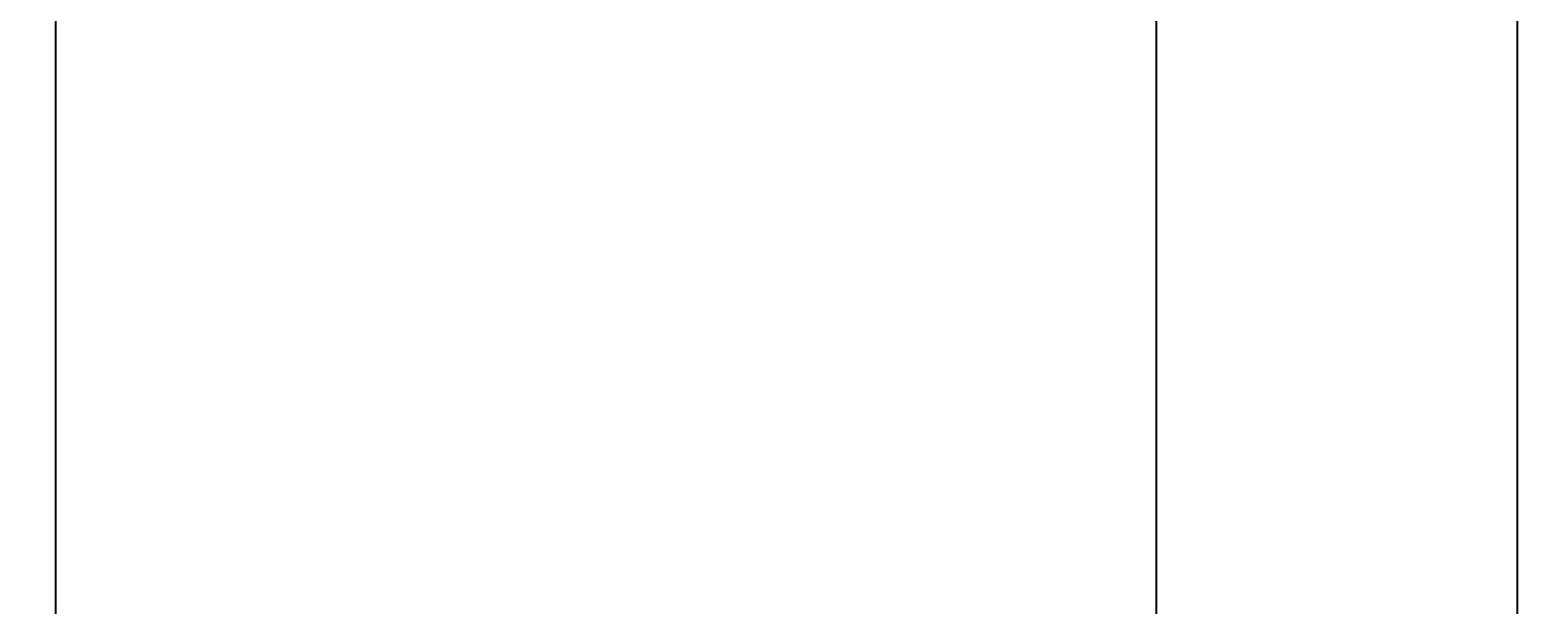
# Model space of a CAD drawing. Units: inches. Extents: x 35362 to 73946, y 43607 to 67532.
# Tile 85 of 134: x 50119 to 51337, y 48329 to 48793. Entities that reach past the tile are written whole.
import ezdxf

# ---------------------------------------------------------------- set-up
doc = ezdxf.new("R2010")
doc.units = ezdxf.units.IN
doc.header["$MEASUREMENT"] = 0
doc.layers.add('A-ANNO-DIMS', color=2, linetype='Continuous', lineweight=18)
doc.styles.get("Standard").update_dxf_attribs({"font": 'arial.ttf'})
doc.dimstyles.get("Standard").update_dxf_attribs({"dimtxt": 0.18, "dimasz": 0.18, "dimexe": 0.18, "dimexo": 0.0625, "dimgap": 0.09, "dimtad": 0, "dimtih": 1, "dimtoh": 1, "dimdec": 4, "dimzin": 0, "dimdsep": 46, "dimtxsty": 'Standard', "dimcen": 0.09, "dimadec": 0, "dimazin": 0, "dimtfac": 1, "dimtdec": 4, "dimtofl": 0, "dimtmove": 0, "dimatfit": 3, "dimfxl": 1, "dimtolj": 1, "dimtzin": 0, "dimarcsym": 0})

# ---------------------------------------------------------------- blocks, each defined once
blk = doc.blocks.new('*D11')
at = {"layer": 'A-ANNO-DIMS', "color": 0, "lineweight": -2, "transparency": 16777216}
for p, q in [((47978.7, 56028.8), (47978.7, 43606.7)), ((53109.8, 56028.8), (53109.8, 43606.7)), ((47978.8, 43606.9), (50543.9, 43606.9)), ((53109.6, 43606.9), (50544.6, 43606.9))]:
    blk.add_line(p, q, dxfattribs=at)
at = {"layer": 'A-ANNO-DIMS', "color": 0, "transparency": 16777216}
for points in [[(47978.8, 43606.9), (47978.8, 43606.8), (47978.7, 43606.9)], [(53109.6, 43606.9), (53109.6, 43606.8), (53109.8, 43606.9)]]:
    blk.add_solid(points, dxfattribs=at)
at = {"layer": 'Defpoints', "color": 0, "transparency": 16777216}
for p in [(47978.7, 56028.8), (53109.8, 56028.8), (53109.8, 43606.9)]:
    blk.add_point(p, dxfattribs=at)
at = {"layer": 'A-ANNO-DIMS', "color": 0, "transparency": 16777216, "insert": (50544.2, 43606.9), "char_height": 0.18, "attachment_point": 5}
blk.add_mtext('\\A1;5131', dxfattribs=at)
blk = doc.blocks.new('*D13')
at = {"layer": 'A-ANNO-DIMS', "color": 0, "lineweight": -2, "transparency": 16777216}
for p, q in [((48373.5, 51694), (48373.5, 43606.7)), ((51029, 51694), (51029, 43606.7)), ((48373.7, 43606.9), (49700.8, 43606.9)), ((51028.9, 43606.9), (49701.7, 43606.9))]:
    blk.add_line(p, q, dxfattribs=at)
at = {"layer": 'A-ANNO-DIMS', "color": 0, "transparency": 16777216}
for points in [[(48373.7, 43606.9), (48373.7, 43606.8), (48373.5, 43606.9)], [(51028.9, 43606.9), (51028.9, 43606.8), (51029, 43606.9)]]:
    blk.add_solid(points, dxfattribs=at)
at = {"layer": 'Defpoints', "color": 0, "transparency": 16777216}
for p in [(48373.5, 51694.1), (51029, 51694.1), (51029, 43606.9)]:
    blk.add_point(p, dxfattribs=at)
at = {"layer": 'A-ANNO-DIMS', "color": 0, "transparency": 16777216, "insert": (49701.3, 43606.9), "char_height": 0.18, "attachment_point": 5}
blk.add_mtext('\\A1;2655.6', dxfattribs=at)
blk = doc.blocks.new('*D17')
at = {"layer": 'A-ANNO-DIMS', "color": 0, "lineweight": -2, "transparency": 16777216}
for p, q in [((49923.3, 61293.2), (49923.3, 43606.7)), ((51913.9, 61293.2), (51913.9, 43606.7)), ((49923.5, 43606.9), (50918.2, 43606.9)), ((51913.8, 43606.9), (50919.1, 43606.9))]:
    blk.add_line(p, q, dxfattribs=at)
at = {"layer": 'A-ANNO-DIMS', "color": 0, "transparency": 16777216}
for points in [[(49923.5, 43606.9), (49923.5, 43606.8), (49923.3, 43606.9)], [(51913.8, 43606.9), (51913.8, 43606.8), (51913.9, 43606.9)]]:
    blk.add_solid(points, dxfattribs=at)
at = {"layer": 'Defpoints', "color": 0, "transparency": 16777216}
for p in [(49923.3, 61293.3), (51913.9, 61293.3), (51913.9, 43606.9)]:
    blk.add_point(p, dxfattribs=at)
at = {"layer": 'A-ANNO-DIMS', "color": 0, "transparency": 16777216, "insert": (50918.6, 43606.9), "char_height": 0.18, "attachment_point": 5}
blk.add_mtext('\\A1;1990.6', dxfattribs=at)
blk = doc.blocks.new('*D67')
at = {"layer": 'A-ANNO-DIMS', "color": 0, "lineweight": -2, "transparency": 16777216}
for p, q in [((56873.5, 53351.5), (35361.8, 53351.5)), ((35361.9, 53351.3), (35361.9, 49400.9)), ((35361.9, 45450.1), (35361.9, 49400.5)), ((53793.6, 45449.9), (35361.8, 45449.9))]:
    blk.add_line(p, q, dxfattribs=at)
at = {"layer": 'A-ANNO-DIMS', "color": 0, "transparency": 16777216}
for points in [[(35361.9, 53351.3), (35362, 53351.3), (35361.9, 53351.5)], [(35361.9, 45450.1), (35362, 45450.1), (35361.9, 45449.9)]]:
    blk.add_solid(points, dxfattribs=at)
at = {"layer": 'Defpoints', "color": 0, "transparency": 16777216}
for p in [(35361.9, 53351.5), (56873.6, 53351.5), (53793.6, 45449.9)]:
    blk.add_point(p, dxfattribs=at)
at = {"layer": 'A-ANNO-DIMS', "color": 0, "transparency": 16777216, "insert": (35361.9, 49400.7), "char_height": 0.18, "attachment_point": 5}
blk.add_mtext('\\A1;7901.6', dxfattribs=at)
blk = doc.blocks.new('*D89')
at = {"layer": 'A-ANNO-DIMS', "color": 0, "lineweight": -2, "transparency": 16777216}
for p, q in [((53707.7, 48897.7), (35361.8, 48897.7)), ((35361.9, 48897.6), (35361.9, 48303.2)), ((35361.9, 47708.4), (35361.9, 48302.8)), ((53707.7, 47708.2), (35361.8, 47708.2))]:
    blk.add_line(p, q, dxfattribs=at)
at = {"layer": 'A-ANNO-DIMS', "color": 0, "transparency": 16777216}
for points in [[(35361.9, 48897.6), (35362, 48897.6), (35361.9, 48897.7)], [(35361.9, 47708.4), (35362, 47708.4), (35361.9, 47708.2)]]:
    blk.add_solid(points, dxfattribs=at)
at = {"layer": 'Defpoints', "color": 0, "transparency": 16777216}
for p in [(53707.8, 48897.7), (35361.9, 47708.2), (53707.8, 47708.2)]:
    blk.add_point(p, dxfattribs=at)
at = {"layer": 'A-ANNO-DIMS', "color": 0, "transparency": 16777216, "insert": (35361.9, 48303), "char_height": 0.18, "attachment_point": 5}
blk.add_mtext('\\A1;1189.5', dxfattribs=at)
blk = doc.blocks.new('*D107')
at = {"layer": 'A-ANNO-DIMS', "color": 0, "lineweight": -2, "transparency": 16777216}
for p, q in [((50139.6, 59850), (50139.6, 43606.7)), ((51320.8, 59850), (51320.8, 43606.7)), ((50139.7, 43606.9), (50729.7, 43606.9)), ((51320.6, 43606.9), (50730.6, 43606.9))]:
    blk.add_line(p, q, dxfattribs=at)
at = {"layer": 'A-ANNO-DIMS', "color": 0, "transparency": 16777216}
for points in [[(50139.7, 43606.9), (50139.7, 43606.8), (50139.6, 43606.9)], [(51320.6, 43606.9), (51320.6, 43606.8), (51320.8, 43606.9)]]:
    blk.add_solid(points, dxfattribs=at)
at = {"layer": 'Defpoints', "color": 0, "transparency": 16777216}
for p in [(50139.6, 59850.1), (51320.8, 59850.1), (51320.8, 43606.9)]:
    blk.add_point(p, dxfattribs=at)
at = {"layer": 'A-ANNO-DIMS', "color": 0, "transparency": 16777216, "insert": (50730.2, 43606.9), "char_height": 0.18, "attachment_point": 5}
blk.add_mtext('\\A1;1181.3', dxfattribs=at)

msp = doc.modelspace()

# ---------------------------------------------------------------- dimensions: what is measured, and where the dimension line sits
at = {"layer": 'A-ANNO-DIMS'}
for base, p1, p2, override, picture, middle in [((51913.931, 43606.859), (49923.307, 61293.286), (51913.931, 61293.286), {"dimdec": 1, "dimlfac": 1, "dimrnd": 0, "dimzin": 0, "dimdsep": 46, "dimlunit": 2}, '*D17', (50918.619, 43606.859)), ((51320.8133, 43606.859), (50139.5627, 59850.0769), (51320.8133, 59850.0769), {"dimdec": 1, "dimlfac": 1, "dimrnd": 0, "dimzin": 0, "dimdsep": 46, "dimlunit": 2}, '*D107', (50730.188, 43606.859)), ((53109.76, 43606.859), (47978.665, 56028.836), (53109.76, 56028.836), {"dimdec": 0, "dimlfac": 1, "dimrnd": 0, "dimzin": 0, "dimdsep": 46, "dimlunit": 2}, '*D11', (50544.212, 43606.859)), ((51029.043, 43606.859), (48373.492, 51694.087), (51029.043, 51694.087), {"dimdec": 1, "dimlfac": 1, "dimrnd": 0, "dimzin": 0, "dimdsep": 46, "dimlunit": 2}, '*D13', (49701.267, 43606.859))]:
    dim = msp.add_linear_dim(base=base, p1=p1, p2=p2, dimstyle='Standard', override=override, dxfattribs=at)
    dim.commit()
    dim.dimension.update_dxf_attribs({"geometry": picture, "text_midpoint": middle})
for base, p1, p2, picture, middle in [((35361.949, 53351.529), (53793.638, 45449.894), (56873.602, 53351.529), '*D67', (35361.949, 49400.712)), ((35361.949, 47708.216), (53707.781, 48897.738), (53707.781, 47708.216), '*D89', (35361.949, 48302.977))]:
    dim = msp.add_linear_dim(base=base, p1=p1, p2=p2, angle=90, dimstyle='Standard', override={"dimdec": 1, "dimlfac": 1, "dimrnd": 0, "dimzin": 0, "dimdsep": 46, "dimlunit": 2}, dxfattribs=at)
    dim.commit()
    dim.dimension.update_dxf_attribs({"geometry": picture, "text_midpoint": middle})

doc.saveas('drawing.dxf')
